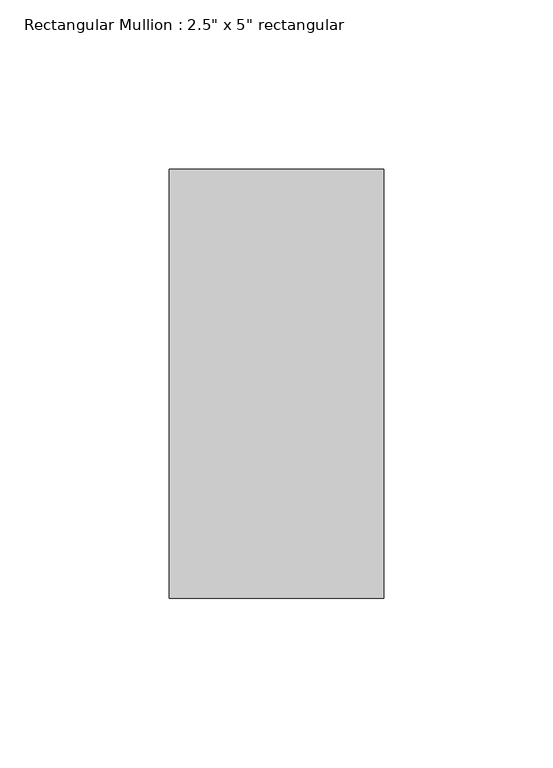
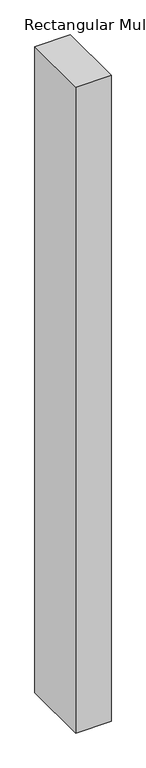
"""IFC4 building model written with IfcOpenShell, lengths in millimetres: member geometry."""

from ifc_helpers import new_model, si_unit, frame, origin, place, context, project, spatial, polyline, outline, extrude, source, transform, mapped, element, save


def member_234fa6b3(model_context):
    return source(origin(), model_context, "Body", "SweptSolid", [
        extrude(outline(polyline([(0.0, 63.5), (0.0, -63.5), (-63.5, -63.5), (-63.5, 63.5), (0.0, 63.5)])), frame((0.0, 0.0, -1226.8199999), z_axis=(0.0, 0.0, 1.0), x_axis=(1.0, 0.0, 0.0)), (0.0, 0.0, 1.0), 1226.8199999),
    ])


if __name__ == "__main__":
    model = new_model("IFC4")
    model_context = context("Model", 3, world=origin())
    ifc_project = project(units=[si_unit("LENGTHUNIT", "METRE", prefix="MILLI")], contexts=[model_context])
    site = spatial("IfcSite", under=ifc_project)
    building = spatial("IfcBuilding", under=site)
    placement = place(None, origin())
    member_shape = member_234fa6b3(model_context)
    element("IfcMember", 1, ObjectType="Rectangular Mullion : 2.5\" x 5\" rectangular", at=placement, inside=building, context=model_context, shape_type="MappedRepresentation", body=[
        mapped(member_shape, transform((0.0, 0.0, 0.0), x_axis=(1.0, 0.0, 0.0), y_axis=(0.0, 1.0, 0.0), z_axis=(0.0, 0.0, 1.0))),
    ])
    save(model, "model.ifc")

# Revit data of these elements
# Type "Rectangular Mullion : 2.5\" x 5\" rectangular"
#   built-in parameter 1007304 = 0.416667 (stored number, unit not read)
#   built-in parameter 1007301 = 0.104167 (stored number, unit not read)
#   built-in parameter 1007300 = 0.104167 (stored number, unit not read)
# Element 1 (IfcMember, "Rectangular Mullion : 2.5\" x 5\" rectangular")
#   Materials on its faces: "BLACK COLOUR"
# Materials
#   "BLACK COLOUR": class "Generic", colour RGB 120 120 120, transparency 0, Cost = 0
